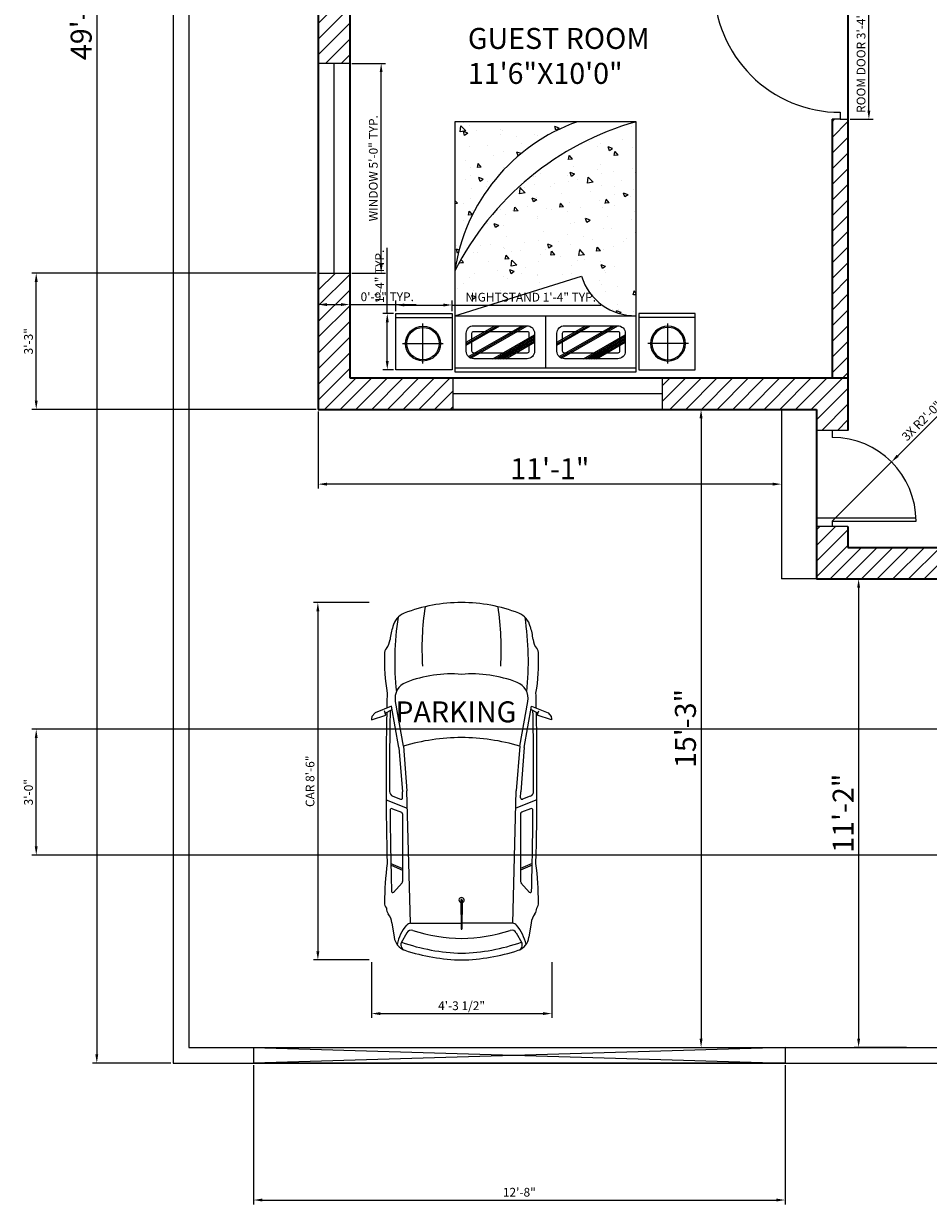
# Model space of a CAD drawing. Units: inches. Extents: x 3618 to 4156, y 1271 to 2023.
# Tile 1 of 5: x 3620 to 3879, y 1297 to 1635. Entities that reach past the tile are written whole.
import ezdxf

# ---------------------------------------------------------------- set-up
doc = ezdxf.new("R2010")
doc.units = ezdxf.units.IN
for name, color, linetype, lineweight in [('A-ANNO-DIMS', 2, 'Continuous', 18), ('A-AREA-IDEN', 7, 'Continuous', 18), ('A-DOOR', 4, 'Continuous', 25), ('A-FLOR-STRS', 7, 'Continuous', 25), ('A-FURN', 8, 'Continuous', 18), ('A-FURN-PATT', 9, 'Continuous', 13), ('A-GLAZ', 4, 'Continuous', 18), ('A-WALL', 7, 'Continuous', 35), ('A-WALL-PATT', 252, 'Continuous', 13), ('C-PROP', 7, 'Continuous', 25), ('C-SITE-VEHI', 8, 'Continuous', 13), ('L-SITE-GATE', 1, 'Continuous', 18)]:
    doc.layers.add(name, color=color, linetype=linetype, lineweight=lineweight)
doc.styles.get("Standard").update_dxf_attribs({"font": 'arial.ttf'})
doc.dimstyles.new('ISO-25', dxfattribs={"dimtxt": 2.5, "dimasz": 2.5, "dimexe": 1.25, "dimexo": 0.625, "dimtad": 1, "dimdec": 0, "dimlunit": 3, "dimtxsty": 'Standard', "dimcen": 2.5, "dimadec": 0, "dimazin": 0, "dimtfac": 1, "dimtdec": 0, "dimtmove": 0, "dimatfit": 3, "dimfxl": 1, "dimarcsym": 0})

# ---------------------------------------------------------------- blocks, each defined once
blk = doc.blocks.new('*D5')
at = {"layer": 'A-ANNO-DIMS', "color": 0, "lineweight": -2, "transparency": 16777216}
for p, q in [((3872.9, 1475.81), (3858, 1475.81)), ((3859.25, 1473.31), (3859.25, 1344.31)), ((3872.9, 1341.81), (3858, 1341.81))]:
    blk.add_line(p, q, dxfattribs=at)
at = {"layer": 'A-ANNO-DIMS', "color": 0, "transparency": 16777216}
for points in [[(3858.83, 1473.31), (3859.67, 1473.31), (3859.25, 1475.81)], [(3858.83, 1344.31), (3859.67, 1344.31), (3859.25, 1341.81)]]:
    blk.add_solid(points, dxfattribs=at)
at = {"layer": 'Defpoints', "color": 0, "transparency": 16777216}
for p in [(3873.53, 1475.81), (3859.25, 1341.81), (3873.53, 1341.81)]:
    blk.add_point(p, dxfattribs=at)
at = {"layer": 'A-ANNO-DIMS', "color": 0, "transparency": 16777216, "insert": (3855.61, 1408.81), "char_height": 6, "attachment_point": 5, "rotation": 90}
blk.add_mtext('11\'-2"', dxfattribs=at)
blk = doc.blocks.new('*D6')
at = {"layer": 'A-ANNO-DIMS', "color": 0, "lineweight": -2, "transparency": 16777216}
for p, q in [((3784.12, 1524.31), (3815.44, 1524.31)), ((3814.19, 1521.81), (3814.19, 1344.31)), ((3784.12, 1341.81), (3815.44, 1341.81))]:
    blk.add_line(p, q, dxfattribs=at)
at = {"layer": 'A-ANNO-DIMS', "color": 0, "transparency": 16777216}
for points in [[(3813.77, 1521.81), (3814.61, 1521.81), (3814.19, 1524.31)], [(3813.77, 1344.31), (3814.61, 1344.31), (3814.19, 1341.81)]]:
    blk.add_solid(points, dxfattribs=at)
at = {"layer": 'Defpoints', "color": 0, "transparency": 16777216}
for p in [(3783.49, 1524.31), (3783.49, 1341.81), (3814.19, 1341.81)]:
    blk.add_point(p, dxfattribs=at)
at = {"layer": 'A-ANNO-DIMS', "color": 0, "transparency": 16777216, "insert": (3810.5, 1433.06), "char_height": 6, "attachment_point": 5, "rotation": 90}
blk.add_mtext('15\'-3"', dxfattribs=at)
blk = doc.blocks.new('*D7')
at = {"layer": 'A-ANNO-DIMS', "color": 0, "lineweight": -2, "transparency": 16777216}
for p, q in [((3704.69, 1523.69), (3704.69, 1501.69)), ((3837.19, 1505.71), (3837.19, 1501.69)), ((3834.69, 1502.94), (3707.19, 1502.94))]:
    blk.add_line(p, q, dxfattribs=at)
at = {"layer": 'A-ANNO-DIMS', "color": 0, "transparency": 16777216}
for points in [[(3707.19, 1503.36), (3707.19, 1502.53), (3704.69, 1502.94)], [(3834.69, 1503.36), (3834.69, 1502.53), (3837.19, 1502.94)]]:
    blk.add_solid(points, dxfattribs=at)
at = {"layer": 'Defpoints', "color": 0, "transparency": 16777216}
for p in [(3704.69, 1524.31), (3837.19, 1506.34), (3704.69, 1502.94)]:
    blk.add_point(p, dxfattribs=at)
at = {"layer": 'A-ANNO-DIMS', "color": 0, "transparency": 16777216, "insert": (3770.94, 1506.58), "char_height": 6, "attachment_point": 5}
blk.add_mtext('11\'-1"', dxfattribs=at)
blk = doc.blocks.new('*D8')
at = {"layer": 'A-ANNO-DIMS', "color": 0, "lineweight": -2, "transparency": 16777216}
for p, q in [((3662.56, 1933.81), (3640.11, 1933.81)), ((3641.36, 1931.31), (3641.36, 1339.81)), ((3662.56, 1337.31), (3640.11, 1337.31))]:
    blk.add_line(p, q, dxfattribs=at)
at = {"layer": 'A-ANNO-DIMS', "color": 0, "transparency": 16777216}
for points in [[(3640.94, 1931.31), (3641.77, 1931.31), (3641.36, 1933.81)], [(3640.94, 1339.81), (3641.77, 1339.81), (3641.36, 1337.31)]]:
    blk.add_solid(points, dxfattribs=at)
at = {"layer": 'Defpoints', "color": 0, "transparency": 16777216}
for p in [(3663.19, 1933.81), (3641.36, 1337.31), (3663.19, 1337.31)]:
    blk.add_point(p, dxfattribs=at)
at = {"layer": 'A-ANNO-DIMS', "color": 0, "transparency": 16777216, "insert": (3637.67, 1635.56), "char_height": 6, "attachment_point": 5, "rotation": 90}
blk.add_mtext('49\'-9"', dxfattribs=at)
blk = doc.blocks.new('A$C2A714640')
for p, q in [((1268, 2029), (1309, 2065)), ((1346, 2068), (1293, 1905)), ((1309, 2065), (1335, 2070)), ((1335, 2070), (1346, 2068)), ((1189, 1839), (1268, 2029)), ((1270, 1913), (1230, 1832)), ((1293, 1905), (1243, 1922)), ((2267, 1901), (2361, 1659)), ((1651, 1703), (1135, 1796)), ((1665, 1754), (1189, 1839)), ((2225, 1825), (2260, 1737)), ((2369, 1829), (2409, 1725)), ((2997, 1847), (3056, 1713)), ((3017, 1845), (3075, 1713)), ((3219, 1718), (3330, 1816)), ((3679, 1836), (3846, 1809)), ((1651, 1703), (2162, 1664)), ((1665, 1754), (2175, 1715)), ((3686, 1623), (2162, 1664)), ((2243, 1713), (2175, 1715)), ((2427, 1713), (3206, 1713)), ((3796, 1664), (3910, 1728)), ((3686, 1622), (3686, 1040)), ((3419, 1043), (3755, 1039)), ((3419, 1028), (3755, 1031)), ((3686, 449), (3686, 1031)), ((3755, 1031), (3755, 1039)), ((3686, 447), (2162, 406)), ((2267, 169), (2361, 412)), ((1651, 367), (1135, 275)), ((1665, 316), (1189, 231)), ((1651, 367), (2162, 406)), ((1665, 316), (2175, 356)), ((2243, 358), (2175, 356)), ((2225, 245), (2260, 333)), ((2369, 241), (2409, 345)), ((2427, 358), (3206, 358)), ((2997, 223), (3056, 358)), ((3017, 225), (3075, 358)), ((3219, 353), (3330, 254)), ((3796, 406), (3910, 342)), ((1189, 231), (1268, 42)), ((1270, 158), (1230, 238)), ((1293, 166), (1243, 148)), ((1346, 2), (1293, 166)), ((3679, 235), (3846, 261)), ((1268, 42), (1309, 5)), ((1309, 5), (1335, 0)), ((1335, 0), (1346, 2))]:
    blk.add_line(p, q)
for centre, radius, start, end in [((585, 1824), 95.5, 87.4739, 128.6871), ((685, -97), 2018, 79.8258, 92.7114), ((2019, -38637), 40539, 88.6181, 91.0712), ((3453, -1618), 3537, 90.0603, 97.4025), ((3453, 1824), 95.5, 51.3129, 92.5261), ((330, 1607), 225, 104.0371, 157.2006), ((670, -1501), 3304, 83.8263, 98.7194), ((499, 1134), 727, 95.9895, 107.9469), ((403, 2052), 197, 275.9895, 308.6871), ((1101, 1602), 197, 79.8299, 158.9468), ((2019, -38637), 40539, 91.1408, 91.3819), ((2019, -38637), 40500, 89.7857, 91.1003), ((2170, 1804), 59, 21.2791, 89.7857), ((2387, 1836), 19.7, 89.6118, 201.2791), ((2105, -39824), 41681, 88.3299, 89.6118), ((3319, 1825), 13.8, 319.5223, 88.2063), ((3517, 1803), 95.5, 51.3129, 92.5261), ((3700, 2031), 197, 231.3129, 264.0105), ((4024, 1301), 484, 101.1159, 130.9804), ((3824, 1631), 180, 18.2803, 83.2196), ((1838, 1035), 1838, 158.994, 180), ((2269, 1152), 1449, 158.9468, 184.6441), ((3873, 1035), 2321, 163.2682, 180), ((2243, 1731), 17.7, 268.4926, 21.2791), ((2427, 1733), 19.7, 201.2791, 270), ((3206, 1733), 19.7, 270, 311.6453), ((3745, 1622), 59, 130.9804, 180), ((3825, 1613), 59, 119.294, 197.2942), ((1860, 992), 2169, 1.135, 19.702), ((3935, 1671), 62.3, 15.1262, 113.3532), ((1889, 989), 2219, 1.2017, 18.3402), ((1822, 985), 2040, 1.3982, 17.3891), ((532, -1813), 3304, 86.544, 98.4137), ((1838, 1035), 1838, 180, 201.006), ((2269, 918), 1449, 175.3559, 201.0532), ((3873, 1035), 2321, 180, 196.7318), ((3419, 1035), 29.7, 13.7603, 346.2397), ((3419, 1035), 7.35, 90, 270), ((1822, 1085), 2040, 342.6109, 358.6018), ((1860, 1078), 2169, 340.298, 358.865), ((1889, 1082), 2219, 341.6598, 358.7983), ((532, 3884), 3304, 261.5863, 273.456), ((3745, 449), 59, 180, 229.0196), ((3825, 458), 59, 162.7058, 240.706), ((330, 464), 225, 202.7994, 255.9629), ((670, 3571), 3304, 261.2806, 276.1737), ((1101, 468), 197, 201.0532, 280.1701), ((2243, 340), 17.7, 338.7209, 91.5074), ((2427, 338), 19.7, 90, 158.7209), ((3206, 338), 19.7, 48.3547, 90), ((4024, 769), 484, 229.0196, 258.8841), ((3824, 440), 180, 276.7804, 341.7197), ((3935, 400), 62.3, 246.6468, 344.8738), ((499, 937), 727, 252.0531, 264.0105), ((403, 18), 197, 51.3129, 84.0105), ((585, 246), 95.5, 231.3129, 272.5261), ((685, 2167), 2018, 267.2886, 280.1742), ((2019, 40707), 40539, 268.6181, 268.8592), ((2019, 40707), 40500, 268.8997, 270.2143), ((2019, 40707), 40539, 268.9288, 271.3819), ((2170, 267), 59, 270.2143, 338.7209), ((2387, 234), 19.7, 158.7209, 270.3882), ((2105, 41894), 41681, 270.3882, 271.6701), ((3453, 3688), 3537, 262.5975, 269.9397), ((3319, 245), 13.8, 271.7937, 40.4777), ((3453, 246), 95.5, 267.4739, 308.6871), ((3517, 267), 95.5, 267.4739, 308.6871), ((3700, 39), 197, 95.9895, 128.6871)]:
    blk.add_arc(centre, radius, start, end)
blk = doc.blocks.new('DOOR-SWING-36')
for p, q in [((-1, -2.25), (-1, 36)), ((0, 0), (0, 36)), ((-38, 0), (-38, 2.25)), ((-36, 0), (-38, 0)), ((-38, 0), (-38, -2.25)), ((2, 0), (0, 0)), ((2, 2.25), (2, -2.25))]:
    blk.add_line(p, q)
blk.add_arc((0, 0), 36, 90, 180)
blk = doc.blocks.new('WINDOW-60X9')
for p, q in [((0, 60), (0, 0)), ((9, 60), (0, 60)), ((4.5, 60), (4.5, 0)), ((9, 0), (9, 60)), ((0, 0), (9, 0))]:
    blk.add_line(p, q)
blk = doc.blocks.new('NIGHTSTAND-16')
for p, q in [((0, 0), (0, 16.11)), ((0, 16.11), (16.11, 16.11)), ((0, 14.98), (16.11, 14.98)), ((16.11, 16.11), (16.11, 0)), ((7.79, 1.77), (7.79, 13.21)), ((1.93, 7.49), (13.52, 7.49)), ((16.11, 0), (0, 0))]:
    blk.add_line(p, q)
for radius in [4.99, 4.63]:
    blk.add_circle((7.79, 7.49), radius)
blk = doc.blocks.new('*D24')
at = {"layer": 'A-ANNO-DIMS', "color": 0, "lineweight": -2, "transparency": 16777216}
for p, q in [((3714.31, 1623.31), (3723.94, 1623.31)), ((3722.69, 1565.81), (3722.69, 1620.81)), ((3714.31, 1563.31), (3723.94, 1563.31))]:
    blk.add_line(p, q, dxfattribs=at)
at = {"layer": 'A-ANNO-DIMS', "color": 0, "transparency": 16777216}
for points in [[(3722.27, 1620.81), (3723.1, 1620.81), (3722.69, 1623.31)], [(3722.27, 1565.81), (3723.1, 1565.81), (3722.69, 1563.31)]]:
    blk.add_solid(points, dxfattribs=at)
at = {"layer": 'Defpoints', "color": 0, "transparency": 16777216}
for p in [(3713.69, 1623.31), (3722.69, 1623.31), (3713.69, 1563.31)]:
    blk.add_point(p, dxfattribs=at)
at = {"layer": 'A-ANNO-DIMS', "color": 0, "transparency": 16777216, "insert": (3720.77, 1593.31), "char_height": 2.5, "attachment_point": 5, "rotation": 90}
blk.add_mtext('WINDOW 5\'-0" TYP.', dxfattribs=at)
blk = doc.blocks.new('*D25')
at = {"layer": 'A-ANNO-DIMS', "color": 0, "lineweight": -2, "transparency": 16777216}
for p, q in [((3704.69, 1562.69), (3704.69, 1553.06)), ((3713.69, 1562.69), (3713.69, 1553.06)), ((3707.19, 1554.31), (3711.19, 1554.31)), ((3713.69, 1554.31), (3732.68, 1554.31))]:
    blk.add_line(p, q, dxfattribs=at)
at = {"layer": 'A-ANNO-DIMS', "color": 0, "transparency": 16777216}
for points in [[(3707.19, 1554.73), (3707.19, 1553.89), (3704.69, 1554.31)], [(3711.19, 1554.73), (3711.19, 1553.89), (3713.69, 1554.31)]]:
    blk.add_solid(points, dxfattribs=at)
at = {"layer": 'Defpoints', "color": 0, "transparency": 16777216}
for p in [(3704.69, 1563.31), (3713.69, 1563.31), (3713.69, 1554.31)]:
    blk.add_point(p, dxfattribs=at)
at = {"layer": 'A-ANNO-DIMS', "color": 0, "transparency": 16777216, "insert": (3724.43, 1556.21), "char_height": 2.5, "attachment_point": 5}
blk.add_mtext('0\'-9" TYP.', dxfattribs=at)
blk = doc.blocks.new('*D32')
at = {"layer": 'A-ANNO-DIMS', "color": 0, "lineweight": -2, "transparency": 16777216}
for p, q in [((3856.81, 1647.31), (3863.44, 1647.31)), ((3862.19, 1609.81), (3862.19, 1644.81)), ((3856.81, 1607.31), (3863.44, 1607.31))]:
    blk.add_line(p, q, dxfattribs=at)
at = {"layer": 'A-ANNO-DIMS', "color": 0, "transparency": 16777216}
for points in [[(3861.77, 1644.81), (3862.6, 1644.81), (3862.19, 1647.31)], [(3861.77, 1609.81), (3862.6, 1609.81), (3862.19, 1607.31)]]:
    blk.add_solid(points, dxfattribs=at)
at = {"layer": 'Defpoints', "color": 0, "transparency": 16777216}
for p in [(3856.19, 1647.31), (3862.19, 1647.31), (3856.19, 1607.31)]:
    blk.add_point(p, dxfattribs=at)
at = {"layer": 'A-ANNO-DIMS', "color": 0, "transparency": 16777216, "insert": (3860.27, 1627.31), "char_height": 2.5, "attachment_point": 5, "rotation": 90}
blk.add_mtext('ROOM DOOR 3\'-4" TYP.', dxfattribs=at)
blk = doc.blocks.new('*D42')
at = {"layer": 'A-ANNO-DIMS', "color": 0, "lineweight": -2, "transparency": 16777216}
for p, q in [((3726.86, 1552.39), (3726.86, 1555.43)), ((3729.36, 1554.18), (3740.46, 1554.18)), ((3742.96, 1552.39), (3742.96, 1555.43)), ((3742.96, 1554.18), (3785.5, 1554.18))]:
    blk.add_line(p, q, dxfattribs=at)
at = {"layer": 'A-ANNO-DIMS', "color": 0, "transparency": 16777216}
for points in [[(3729.36, 1554.6), (3729.36, 1553.76), (3726.86, 1554.18)], [(3740.46, 1554.6), (3740.46, 1553.76), (3742.96, 1554.18)]]:
    blk.add_solid(points, dxfattribs=at)
at = {"layer": 'Defpoints', "color": 0, "transparency": 16777216}
for p in [(3742.96, 1554.18), (3726.86, 1551.76), (3742.96, 1551.76)]:
    blk.add_point(p, dxfattribs=at)
at = {"layer": 'A-ANNO-DIMS', "color": 0, "transparency": 16777216, "insert": (3765.48, 1556.1), "char_height": 2.5, "attachment_point": 5}
blk.add_mtext('NIGHTSTAND 1\'-4" TYP.', dxfattribs=at)
blk = doc.blocks.new('*D43')
at = {"layer": 'A-ANNO-DIMS', "color": 0, "lineweight": -2, "transparency": 16777216}
for p, q in [((3724.44, 1551.76), (3724.44, 1570.52)), ((3726.23, 1551.76), (3723.19, 1551.76)), ((3724.44, 1538.16), (3724.44, 1549.26)), ((3726.23, 1535.66), (3723.19, 1535.66))]:
    blk.add_line(p, q, dxfattribs=at)
at = {"layer": 'A-ANNO-DIMS', "color": 0, "transparency": 16777216}
for points in [[(3724.02, 1549.26), (3724.86, 1549.26), (3724.44, 1551.76)], [(3724.02, 1538.16), (3724.86, 1538.16), (3724.44, 1535.66)]]:
    blk.add_solid(points, dxfattribs=at)
at = {"layer": 'Defpoints', "color": 0, "transparency": 16777216}
for p in [(3724.44, 1551.76), (3726.86, 1551.76), (3726.86, 1535.66)]:
    blk.add_point(p, dxfattribs=at)
at = {"layer": 'A-ANNO-DIMS', "color": 0, "transparency": 16777216, "insert": (3722.56, 1562.39), "char_height": 2.5, "attachment_point": 5, "rotation": 90}
blk.add_mtext('1\'-4" TYP.', dxfattribs=at)
blk = doc.blocks.new('*D48')
at = {"layer": 'A-ANNO-DIMS', "color": 0, "lineweight": -2, "transparency": 16777216}
for p, q in [((3719.3, 1469.06), (3703.34, 1469.06)), ((3704.59, 1466.56), (3704.59, 1369.32)), ((3719.3, 1366.82), (3703.34, 1366.82))]:
    blk.add_line(p, q, dxfattribs=at)
at = {"layer": 'A-ANNO-DIMS', "color": 0, "transparency": 16777216}
for points in [[(3704.17, 1466.56), (3705.01, 1466.56), (3704.59, 1469.06)], [(3704.17, 1369.32), (3705.01, 1369.32), (3704.59, 1366.82)]]:
    blk.add_solid(points, dxfattribs=at)
at = {"layer": 'Defpoints', "color": 0, "transparency": 16777216}
for p in [(3719.92, 1469.06), (3704.59, 1366.82), (3719.92, 1366.82)]:
    blk.add_point(p, dxfattribs=at)
at = {"layer": 'A-ANNO-DIMS', "color": 0, "transparency": 16777216, "insert": (3702.67, 1417.94), "char_height": 2.5, "attachment_point": 5, "rotation": 90}
blk.add_mtext('CAR 8\'-6"', dxfattribs=at)
blk = doc.blocks.new('*D49')
at = {"layer": 'A-ANNO-DIMS', "color": 0, "lineweight": -2, "transparency": 16777216}
for p, q in [((3719.92, 1366.2), (3719.92, 1350.24)), ((3771.46, 1366.2), (3771.46, 1350.24)), ((3722.42, 1351.49), (3768.96, 1351.49))]:
    blk.add_line(p, q, dxfattribs=at)
at = {"layer": 'A-ANNO-DIMS', "color": 0, "transparency": 16777216}
for points in [[(3722.42, 1351.91), (3722.42, 1351.07), (3719.92, 1351.49)], [(3768.96, 1351.91), (3768.96, 1351.07), (3771.46, 1351.49)]]:
    blk.add_solid(points, dxfattribs=at)
at = {"layer": 'Defpoints', "color": 0, "transparency": 16777216}
for p in [(3719.92, 1366.82), (3771.46, 1366.82), (3771.46, 1351.49)]:
    blk.add_point(p, dxfattribs=at)
at = {"layer": 'A-ANNO-DIMS', "color": 0, "transparency": 16777216, "insert": (3745.69, 1353.41), "char_height": 2.5, "attachment_point": 5}
blk.add_mtext('4\'-3 1/2"', dxfattribs=at)
blk = doc.blocks.new('*D52')
at = {"layer": 'A-ANNO-DIMS', "color": 0, "lineweight": -2, "transparency": 16777216}
for p, q in [((3927.56, 1432.81), (3622.79, 1432.81)), ((3624.04, 1399.31), (3624.04, 1430.31)), ((3927.56, 1396.81), (3622.79, 1396.81))]:
    blk.add_line(p, q, dxfattribs=at)
at = {"layer": 'A-ANNO-DIMS', "color": 0, "transparency": 16777216}
for points in [[(3623.62, 1430.31), (3624.45, 1430.31), (3624.04, 1432.81)], [(3623.62, 1399.31), (3624.45, 1399.31), (3624.04, 1396.81)]]:
    blk.add_solid(points, dxfattribs=at)
at = {"layer": 'Defpoints', "color": 0, "transparency": 16777216}
for p in [(3624.04, 1432.81), (3928.19, 1432.81), (3928.19, 1396.81)]:
    blk.add_point(p, dxfattribs=at)
at = {"layer": 'A-ANNO-DIMS', "color": 0, "transparency": 16777216, "insert": (3622.14, 1414.81), "char_height": 2.5, "attachment_point": 5, "rotation": 90}
blk.add_mtext('3\'-0"', dxfattribs=at)
blk = doc.blocks.new('*D54')
at = {"layer": 'A-ANNO-DIMS', "color": 0, "lineweight": -2, "transparency": 16777216}
for p, q in [((3686.19, 1336.69), (3686.19, 1296.91)), ((3838.24, 1336.69), (3838.24, 1296.91)), ((3688.69, 1298.16), (3835.74, 1298.16))]:
    blk.add_line(p, q, dxfattribs=at)
at = {"layer": 'A-ANNO-DIMS', "color": 0, "transparency": 16777216}
for points in [[(3688.69, 1298.58), (3688.69, 1297.74), (3686.19, 1298.16)], [(3835.74, 1298.58), (3835.74, 1297.74), (3838.24, 1298.16)]]:
    blk.add_solid(points, dxfattribs=at)
at = {"layer": 'Defpoints', "color": 0, "transparency": 16777216}
for p in [(3686.19, 1337.31), (3838.24, 1337.31), (3838.24, 1298.16)]:
    blk.add_point(p, dxfattribs=at)
at = {"layer": 'A-ANNO-DIMS', "color": 0, "transparency": 16777216, "insert": (3762.21, 1300.06), "char_height": 2.5, "attachment_point": 5}
blk.add_mtext('12\'-8"', dxfattribs=at)
blk = doc.blocks.new('*D58')
at = {"layer": 'A-ANNO-DIMS', "color": 0, "lineweight": -2, "transparency": 16777216}
for p, q in [((3704.06, 1563.31), (3622.79, 1563.31)), ((3624.04, 1526.81), (3624.04, 1560.81)), ((3704.06, 1524.31), (3622.79, 1524.31))]:
    blk.add_line(p, q, dxfattribs=at)
at = {"layer": 'A-ANNO-DIMS', "color": 0, "transparency": 16777216}
for points in [[(3623.62, 1560.81), (3624.45, 1560.81), (3624.04, 1563.31)], [(3623.62, 1526.81), (3624.45, 1526.81), (3624.04, 1524.31)]]:
    blk.add_solid(points, dxfattribs=at)
at = {"layer": 'Defpoints', "color": 0, "transparency": 16777216}
for p in [(3624.04, 1563.31), (3704.69, 1563.31), (3704.69, 1524.31)]:
    blk.add_point(p, dxfattribs=at)
at = {"layer": 'A-ANNO-DIMS', "color": 0, "transparency": 16777216, "insert": (3622.14, 1543.81), "char_height": 2.5, "attachment_point": 5, "rotation": 90}
blk.add_mtext('3\'-3"', dxfattribs=at)
blk = doc.blocks.new('*D62')
at = {"layer": 'A-ANNO-DIMS', "color": 0, "lineweight": -2, "transparency": 16777216}
for p, q in [((3884.38, 1525), (3870.43, 1511.05)), ((3851.69, 1492.31), (3868.66, 1509.28))]:
    blk.add_line(p, q, dxfattribs=at)
at = {"layer": 'A-ANNO-DIMS', "color": 0, "transparency": 16777216}
blk.add_solid([(3870.13, 1511.34), (3870.72, 1510.75), (3868.66, 1509.28)], dxfattribs=at)
at = {"layer": 'Defpoints', "color": 0, "transparency": 16777216}
for p in [(3868.66, 1509.28), (3851.69, 1492.31)]:
    blk.add_point(p, dxfattribs=at)
at = {"layer": 'A-ANNO-DIMS', "color": 0, "transparency": 16777216, "insert": (3877.5, 1520.81), "char_height": 2.5, "attachment_point": 5, "rotation": 45.0011}
blk.add_mtext('3X R2\'-0"', dxfattribs=at)

msp = doc.modelspace()

# ---------------------------------------------------------------- hatches: boundary and pattern name
at = {"layer": 'A-FURN-PATT'}
h = msp.add_hatch(dxfattribs=at)
h.set_pattern_fill('AR-CONC', color=256, scale=0.071583, angle=360, style=0)
h.set_pattern_definition([(130, (4407.12, -2224.239), (-13.04127, -1.140963), [1.36365, -15.000153]), (185, (4407.12, -2224.239), (2.522776, 13.67635), [1.09092, -12.000122]), (79.549, (4406.033, -2224.334), (-10.51854, 12.535324), [1.158924, -12.74816]), (133.8158, (4407.12, -2220.603), (-19.40457, -3.0095), [2.04548, -22.50023]), (83.3644, (4405.503, -2220.854), (-16.99403, 17.71139), [1.73839, -19.12224]), (188.816, (4407.12, -2220.603), (-16.99406, 17.71136), [1.63638, -18.00018]), (159, (4405.301, -2221.512), (-10.853, -7.32044), [1.36365, -15.000153]), (214, (4405.301, -2221.512), (-4.423956, 13.18467), [1.09092, -12.000122]), (108.5486, (4404.397, -2222.122), (-15.276927, 5.86426), [1.158924, -12.74816]), (142.5, (4407.1196, -2224.239), (-0.2210905, 6.0526773), [0, -11.854666, 0, -12.181943, 0, -12.045577]), (172.5, (4407.1196, -2224.239), (-4.783131, 7.171195), [0, -6.945525, 0, -11.581936, 0, -4.590956]), (212.5, (4411.174, -2224.239), (-9.70594, -0.410079), [0, -4.545501, 0, -14.181963, 0, -18.818374]), (222.5, (4412.992, -2224.239), (-10.603486, 1.820097), [0, -5.909151, 0, -9.418278, 0, -13.363773])])
edge = h.paths.add_edge_path()
edge.add_ellipse((3795.31, 1567.11), major_axis=(11.32, 11.32), ratio=1, start_angle=151.9547, end_angle=223.8468)
edge.add_line((3794.99, 1551.11), (3795.63, 1551.11))
edge.add_line((3795.63, 1551.11), (3795.63, 1606.62))
edge.add_ellipse((3818.43, 1526.11), major_axis=(59.17, 59.17), ratio=1, start_angle=60.8086, end_angle=108.2045)
edge.add_line((3743.73, 1563.83), (3743.73, 1551.11))
edge.add_line((3743.73, 1551.11), (3780, 1562.44))
edge = h.paths.add_edge_path()
edge.add_line((3778.89, 1606.62), (3743.73, 1606.62))
edge.add_line((3743.73, 1606.62), (3743.73, 1563.83))
edge.add_ellipse((3796.71, 1556.14), major_axis=(-37.85, 37.85), ratio=1, start_angle=-25.5572, end_angle=36.7417, ccw=False)
h = msp.add_hatch(dxfattribs=at)
h.set_pattern_fill('ANSI31', color=256, scale=0.11269752, angle=-15.041628, style=0)
h.paths.add_polyline_path([(3747.03, 1542.6), (3747.03, 1543.63), (3755.04, 1548.25), (3756.83, 1548.25)])
h = msp.add_hatch(dxfattribs=at)
h.set_pattern_fill('ANSI31', color=256, scale=0.11276227, angle=-15.041628, style=0)
h.paths.add_polyline_path([(3748.45, 1538.94), (3748.34, 1538.98), (3748.22, 1539.04), (3748.09, 1539.1), (3747.98, 1539.18), (3747.87, 1539.26), (3747.76, 1539.35), (3747.66, 1539.44), (3747.62, 1539.49), (3762.83, 1548.25), (3764.42, 1548.25), (3764.49, 1548.25), (3764.56, 1548.25), (3764.6, 1548.24)])
h = msp.add_hatch(dxfattribs=at)
h.set_pattern_fill('ANSI31', color=256, scale=0.11271331, angle=-15.041628, style=0)
h.paths.add_polyline_path([(3772.98, 1542.6), (3772.98, 1543.63), (3780.99, 1548.25), (3782.78, 1548.25)])
h = msp.add_hatch(dxfattribs=at)
h.set_pattern_fill('ANSI31', color=256, scale=0.11270326, angle=-15.041628, style=0)
h.paths.add_polyline_path([(3774.4, 1538.94), (3774.37, 1538.95), (3774.3, 1538.97), (3774.24, 1539), (3774.18, 1539.03), (3774.12, 1539.06), (3774.05, 1539.1), (3773.99, 1539.13), (3773.94, 1539.17), (3773.88, 1539.21), (3773.82, 1539.25), (3773.77, 1539.3), (3773.71, 1539.34), (3773.66, 1539.39), (3773.61, 1539.44), (3773.56, 1539.48), (3788.78, 1548.25), (3790.37, 1548.25), (3790.44, 1548.25), (3790.51, 1548.25), (3790.55, 1548.24)])
h = msp.add_hatch(dxfattribs=at)
h.set_pattern_fill('ANSI31', color=256, scale=0.11816216, angle=-15.041628, style=0)
h.paths.add_polyline_path([(3758.56, 1538.81), (3754.43, 1538.81), (3766.56, 1545.8), (3766.56, 1543.42)])
h = msp.add_hatch(dxfattribs=at)
h.set_pattern_fill('ANSI31', color=256, scale=0.1181255, angle=-15.041628, style=0)
h.paths.add_polyline_path([(3784.51, 1538.81), (3780.38, 1538.81), (3792.51, 1545.8), (3792.51, 1543.42)])
at = {"layer": 'A-WALL-PATT'}
h = msp.add_hatch(dxfattribs=at)
h.set_pattern_fill('ANSI31', color=256)
h.paths.add_polyline_path([(4115.69, 1933.81), (3704.69, 1933.81), (3704.69, 1885.81), (3713.69, 1885.81), (3713.69, 1924.81), (4115.69, 1924.81)])
h.paths.add_polyline_path([(3886.19, 1924.81), (3881.69, 1924.81), (3881.69, 1786.81), (3875.69, 1786.81), (3875.69, 1782.31), (3892.19, 1782.31), (3892.19, 1786.81), (3886.19, 1786.81)])
h.paths.add_polyline_path([(3763.69, 1784.56), (3763.69, 1786.81), (3713.69, 1786.81), (3713.69, 1782.31), (3763.69, 1782.31)], flags=17)
h.paths.add_polyline_path([(3713.69, 1825.81), (3704.69, 1825.81), (3704.69, 1764.31), (3713.69, 1764.31)])
h.paths.add_polyline_path([(3802.19, 1782.31), (3835.69, 1782.31), (3835.69, 1784.56), (3835.69, 1786.81), (3791.69, 1786.81), (3791.69, 1782.31), (3797.69, 1782.31), (3797.69, 1722.31), (3713.69, 1722.31), (3713.69, 1717.81), (3797.69, 1717.81), (3797.69, 1657.81), (3791.69, 1657.81), (3791.69, 1653.31), (3851.69, 1653.31), (3851.69, 1647.31), (3856.19, 1647.31), (3856.19, 1657.81), (3802.19, 1657.81)])
h.paths.add_polyline_path([(3713.69, 1740.31), (3704.69, 1740.31), (3704.69, 1699.81), (3713.69, 1699.81)])
h.paths.add_polyline_path([(3713.69, 1675.81), (3704.69, 1675.81), (3704.69, 1623.31), (3713.69, 1623.31)])
h.paths.add_polyline_path([(3743.18, 1533.31), (3713.69, 1533.31), (3713.69, 1563.31), (3704.69, 1563.31), (3704.69, 1524.31), (3743.18, 1524.31)])
h.paths.add_polyline_path([(3856.19, 1533.31), (3803.18, 1533.31), (3803.18, 1524.31), (3847.19, 1524.31), (3847.19, 1518.31), (3856.19, 1518.31)])
h.paths.add_polyline_path([(3856.19, 1607.31), (3853.94, 1607.31), (3851.69, 1607.31), (3851.69, 1533.31), (3856.19, 1533.31)])
h.paths.add_polyline_path([(3763.69, 1655.56), (3763.69, 1657.81), (3713.69, 1657.81), (3713.69, 1653.31), (3763.69, 1653.31)], flags=17)
h.paths.add_polyline_path([(4063.19, 1670.56), (4054.19, 1670.56), (4054.19, 1645.31), (3940.98, 1645.31), (3940.98, 1640.81), (4054.19, 1640.81), (4054.19, 1592.81), (4063.19, 1592.81)])
h.paths.add_polyline_path([(4063.19, 1532.81), (4054.19, 1532.81), (4054.19, 1454.31), (4063.19, 1454.31)])
h.paths.add_polyline_path([(4054.19, 1484.81), (3985.19, 1484.81), (3985.19, 1475.81), (4054.19, 1475.81)])
h.paths.add_polyline_path([(3925.19, 1484.81), (3856.19, 1484.81), (3856.19, 1490.81), (3847.19, 1490.81), (3847.19, 1475.81), (3925.19, 1475.81)])
h.paths.add_polyline_path([(4063.19, 1396.81), (3928.19, 1396.81), (3928.19, 1387.81), (4063.19, 1387.81)])
h.paths.add_polyline_path([(4063.19, 1418.31), (4054.19, 1418.31), (4054.19, 1396.81), (4063.19, 1396.81)])
h.paths.add_polyline_path([(4063.19, 1790.42), (4054.19, 1790.42), (4054.19, 1786.81), (3932.19, 1786.81), (3932.19, 1784.56), (3932.19, 1782.31), (4054.19, 1782.31), (4054.19, 1771.81), (4063.19, 1771.81)])
h.paths.add_polyline_path([(4070.69, 1840.81), (4058.69, 1840.81), (4058.69, 1890.81), (4056.44, 1890.81), (4054.19, 1890.81), (4054.19, 1826.42), (4063.19, 1826.42), (4063.19, 1831.81), (4070.69, 1831.81)])
h.paths.add_polyline_path([(4115.69, 1924.81), (4106.69, 1924.81), (4106.69, 1840.81), (4094.69, 1840.81), (4094.69, 1831.81), (4115.69, 1831.81)])
h.paths.add_polyline_path([(4063.19, 1731.81), (4058.69, 1731.81), (4054.19, 1731.81), (4054.19, 1706.56), (4063.19, 1706.56)])

# ---------------------------------------------------------------- linework, layer by layer
at = {"layer": 'A-DOOR'}
for p, q in [((3856.19, 1518.31), (3847.19, 1518.31)), ((3851.69, 1518.31), (3851.69, 1516.31)), ((3847.19, 1493.31), (3875.69, 1493.31)), ((3856.19, 1490.81), (3847.19, 1490.81)), ((3851.69, 1492.31), (3851.69, 1490.81)), ((3851.69, 1492.31), (3875.69, 1492.31))]:
    msp.add_line(p, q, dxfattribs=at)
msp.add_arc((3851.69, 1492.31), 24, 360, 90, dxfattribs=at)
at = {"layer": 'A-FLOR-STRS'}
for p in [(3837.19, 1524.31), (3847.19, 1475.81)]:
    msp.add_line(p, (3837.19, 1475.81), dxfattribs=at)
at = {"layer": 'A-FURN'}
for p, q in [((3743.73, 1606.62), (3743.73, 1535.04)), ((3795.63, 1606.62), (3743.73, 1606.62)), ((3795.63, 1535.04), (3795.63, 1606.62)), ((3743.73, 1551.11), (3780, 1562.44)), ((3743.73, 1551.11), (3795.63, 1551.11)), ((3769.68, 1551.11), (3769.68, 1536.21)), ((3743.73, 1536.21), (3795.63, 1536.21)), ((3743.73, 1535.04), (3795.63, 1535.04))]:
    msp.add_line(p, q, dxfattribs=at)
for points in [[(3764.42, 1538.81), (3749.18, 1538.81, -0.414214), (3747.03, 1540.96), (3747.03, 1546.11, -0.414214), (3749.18, 1548.25), (3764.42, 1548.25, -0.414214), (3766.56, 1546.11), (3766.56, 1540.96, -0.414214)], [(3790.37, 1538.81), (3775.13, 1538.81, -0.414214), (3772.98, 1540.96), (3772.98, 1546.11, -0.414214), (3775.13, 1548.25), (3790.37, 1548.25, -0.414214), (3792.51, 1546.11), (3792.51, 1540.96, -0.414214)], [(3764.42, 1540.42), (3749.18, 1540.42, -0.414214), (3748.64, 1540.96), (3748.64, 1546.11, -0.414214), (3749.18, 1546.64), (3764.42, 1546.64, -0.414214), (3764.95, 1546.11), (3764.95, 1540.96, -0.414214)], [(3790.37, 1540.42), (3775.13, 1540.42, -0.414214), (3774.59, 1540.96), (3774.59, 1546.11, -0.414214), (3775.13, 1546.64), (3790.37, 1546.64, -0.414214), (3790.9, 1546.11), (3790.9, 1540.96, -0.414214)]]:
    msp.add_lwpolyline(points, format="xyb", close=True, dxfattribs=at)
for centre, radius, start, end in [((3818.43, 1526.11), 83.68, 105.8086, 153.2045), ((3796.71, 1556.14), 53.53, 109.4428, 171.7417), ((3795.31, 1567.11), 16, 196.9547, 271.1532)]:
    msp.add_arc(centre, radius, start, end, dxfattribs=at)
at = {"layer": 'A-WALL'}
for p, q in [((3704.69, 1933.81), (3704.69, 1524.31)), ((3713.69, 1924.81), (3713.69, 1533.31)), ((3856.19, 1657.81), (3856.19, 1518.31)), ((3851.69, 1607.31), (3851.69, 1533.31)), ((3713.69, 1533.31), (3856.19, 1533.31)), ((3704.69, 1524.31), (3847.19, 1524.31)), ((3847.19, 1524.31), (3847.19, 1475.81)), ((3856.19, 1490.81), (3856.19, 1484.81)), ((3856.19, 1484.81), (4054.19, 1484.81)), ((3847.19, 1475.81), (4054.19, 1475.81))]:
    msp.add_line(p, q, dxfattribs=at)
at = {"layer": 'C-PROP'}
for p, q in [((3663.19, 1933.81), (3663.19, 1524.31)), ((3667.69, 1933.81), (3667.69, 1524.31)), ((3663.19, 1524.31), (3663.19, 1341.81)), ((3667.69, 1524.31), (3667.69, 1341.81)), ((3663.19, 1341.81), (3663.19, 1337.31)), ((3667.69, 1341.81), (3667.69, 1341.81)), ((3667.69, 1341.81), (3704.69, 1341.81)), ((3704.69, 1341.81), (4111.19, 1341.81)), ((3663.19, 1337.31), (3667.69, 1337.31)), ((3667.69, 1337.31), (3704.69, 1337.31)), ((3704.69, 1337.31), (4115.69, 1337.31))]:
    msp.add_line(p, q, dxfattribs=at)
at = {"layer": 'L-SITE-GATE'}
for p, q in [((3686.19, 1341.81), (3686.19, 1337.31)), ((3838.24, 1341.81), (3686.19, 1337.31)), ((3686.19, 1341.81), (3838.24, 1337.31)), ((3686.19, 1341.81), (3686.19, 1337.31)), ((3686.19, 1341.81), (3838.24, 1341.81)), ((3838.24, 1341.81), (3838.24, 1337.31)), ((3838.24, 1341.81), (3838.24, 1337.31)), ((3838.24, 1337.31), (3686.19, 1337.31))]:
    msp.add_line(p, q, dxfattribs=at)

# ---------------------------------------------------------------- block references
at = {"layer": 'A-DOOR', "rotation": 90.00000000000087}
msp.add_blockref('DOOR-SWING-36', (3853.94, 1645.31), dxfattribs=at)
at = {"layer": 'A-FURN'}
msp.add_blockref('NIGHTSTAND-16', (3726.86, 1535.66), dxfattribs=at)
at = {"layer": 'A-FURN', "extrusion": (0, 0, -1), "zscale": -1}
msp.add_blockref('NIGHTSTAND-16', (-3812.51, 1535.66), dxfattribs=at)
at = {"layer": 'A-GLAZ'}
msp.add_blockref('WINDOW-60X9', (3704.69, 1563.31), dxfattribs=at)
at = {"layer": 'A-GLAZ', "rotation": 270.0000000000025}
msp.add_blockref('WINDOW-60X9', (3743.18, 1533.31), dxfattribs=at)
at = {"layer": 'C-SITE-VEHI', "xscale": 0.0248913959350011, "yscale": 0.0248913959350011, "zscale": 0.0248913959350011, "rotation": 270}
msp.add_blockref('A$C2A714640', (3719.92, 1469.06), dxfattribs=at)

# ---------------------------------------------------------------- texts
at = {"layer": 'A-AREA-IDEN', "char_height": 6, "attachment_point": 1}
for s, insert in [('GUEST ROOM\\P11\'6"X10\'0"', (3747.49, 1633.44)), ('PARKING', (3726.76, 1440.8))]:
    msp.add_mtext(s, dxfattribs=dict(at, insert=insert))

# ---------------------------------------------------------------- dimensions: what is measured, and where the dimension line sits
at = {"layer": 'A-ANNO-DIMS'}
for base, p1, p2, override, picture, middle in [((3641.35613458, 1337.31015181), (3663.18781808, 1933.81015181), (3663.18781808, 1337.31015181), {"dimtxt": 6, "dimclrd": 0, "dimclre": 0, "dimclrt": 0}, '*D8', (3637.66769666, 1635.56015181)), ((3624.04, 1563.31), (3704.69, 1524.31), (3704.69, 1563.31), {"dimdec": 1, "dimlfac": 1, "dimrnd": 0, "dimzin": 1, "dimdsep": 46, "dimlunit": 4, "dimfrac": 2}, '*D58', (3622.14, 1543.81)), ((3814.18945307, 1341.81015181), (3783.49037408, 1524.31015181), (3783.49037408, 1341.81015181), {"dimtxt": 6, "dimclrd": 0, "dimclre": 0, "dimclrt": 0}, '*D6', (3810.49896876, 1433.06015181)), ((3859.25, 1341.81), (3873.53, 1475.81), (3873.53, 1341.81), {"dimtxt": 6, "dimclrd": 0, "dimclre": 0, "dimclrt": 0}, '*D5', (3855.61, 1408.81)), ((3624.04, 1432.81), (3928.19, 1396.81), (3928.19, 1432.81), {"dimdec": 1, "dimlfac": 1, "dimrnd": 0, "dimzin": 1, "dimdsep": 46, "dimlunit": 4, "dimfrac": 2}, '*D52', (3622.14, 1414.81))]:
    dim = msp.add_linear_dim(base=base, p1=p1, p2=p2, angle=90, dimstyle='ISO-25', override=override, dxfattribs=at)
    dim.commit()
    dim.dimension.update_dxf_attribs({"geometry": picture, "text_midpoint": middle})
for base, p1, p2, angle, text, picture, middle in [((3862.19, 1647.31), (3856.19, 1607.31), (3856.19, 1647.31), 90, 'ROOM DOOR <> TYP.', '*D32', (3860.27, 1627.31)), ((3722.69, 1623.31), (3713.69, 1563.31), (3713.69, 1623.31), 90, 'WINDOW <> TYP.', '*D24', (3720.77, 1593.31)), ((3724.44, 1551.76), (3726.86, 1535.66), (3726.86, 1551.76), 90, '<> TYP.', '*D43', (3722.56, 1562.39)), ((3704.59, 1366.82), (3719.92, 1469.06), (3719.92, 1366.82), 270, 'CAR <>', '*D48', (3702.67, 1417.94))]:
    dim = msp.add_linear_dim(base=base, p1=p1, p2=p2, angle=angle, text=text, dimstyle='ISO-25', override={"dimdec": 1, "dimlfac": 1, "dimrnd": 0, "dimzin": 1, "dimdsep": 46, "dimlunit": 4, "dimfrac": 2}, dxfattribs=at)
    dim.commit()
    dim.dimension.update_dxf_attribs({"geometry": picture, "text_midpoint": middle})
for base, p1, p2, text, picture, middle in [((3713.69, 1554.31), (3704.69, 1563.31), (3713.69, 1563.31), '<> TYP.', '*D25', (3724.43, 1556.21)), ((3742.96, 1554.18), (3726.86, 1551.76), (3742.96, 1551.76), 'NIGHTSTAND <> TYP.', '*D42', (3765.48, 1556.1))]:
    dim = msp.add_linear_dim(base=base, p1=p1, p2=p2, text=text, dimstyle='ISO-25', override={"dimdec": 1, "dimlfac": 1, "dimrnd": 0, "dimzin": 1, "dimdsep": 46, "dimlunit": 4, "dimfrac": 2}, dxfattribs=at)
    dim.commit()
    dim.dimension.update_dxf_attribs({"geometry": picture, "text_midpoint": middle})
dim = msp.add_radius_dim(center=(3851.69, 1492.31), mpoint=(3868.66, 1509.28), text='3X <>', dimstyle='ISO-25', override={"dimdec": 1, "dimlfac": 1, "dimrnd": 0, "dimzin": 1, "dimdsep": 46, "dimlunit": 4, "dimfrac": 2}, dxfattribs=at)
dim.commit()
dim.dimension.update_dxf_attribs({"geometry": '*D62', "text_midpoint": (3878.84, 1519.46), "dimtype": 164})
for base, p1, p2, override, picture, middle in [((3704.68781808, 1502.94446085), (3837.18781808, 1506.33686094), (3704.68781808, 1524.31015181), {"dimtxt": 6, "dimclrd": 0, "dimclre": 0, "dimclrt": 0}, '*D7', (3770.93781808, 1506.58173916)), ((3771.46, 1351.49), (3719.92, 1366.82), (3771.46, 1366.82), {"dimdec": 1, "dimlfac": 1, "dimrnd": 0, "dimzin": 1, "dimdsep": 46, "dimlunit": 4, "dimfrac": 2}, '*D49', (3745.69, 1353.41)), ((3838.2353, 1298.1602), (3686.1878, 1337.3102), (3838.2353, 1337.3102), {"dimdec": 1, "dimlfac": 1, "dimrnd": 0, "dimzin": 1, "dimdsep": 46, "dimlunit": 4, "dimfrac": 2}, '*D54', (3762.2116, 1300.0616))]:
    dim = msp.add_linear_dim(base=base, p1=p1, p2=p2, dimstyle='ISO-25', override=override, dxfattribs=at)
    dim.commit()
    dim.dimension.update_dxf_attribs({"geometry": picture, "text_midpoint": middle})

doc.saveas('drawing.dxf')
